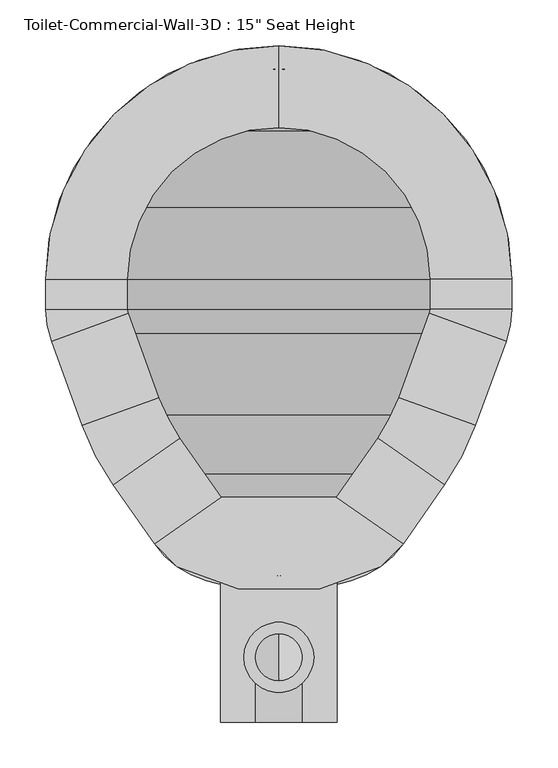
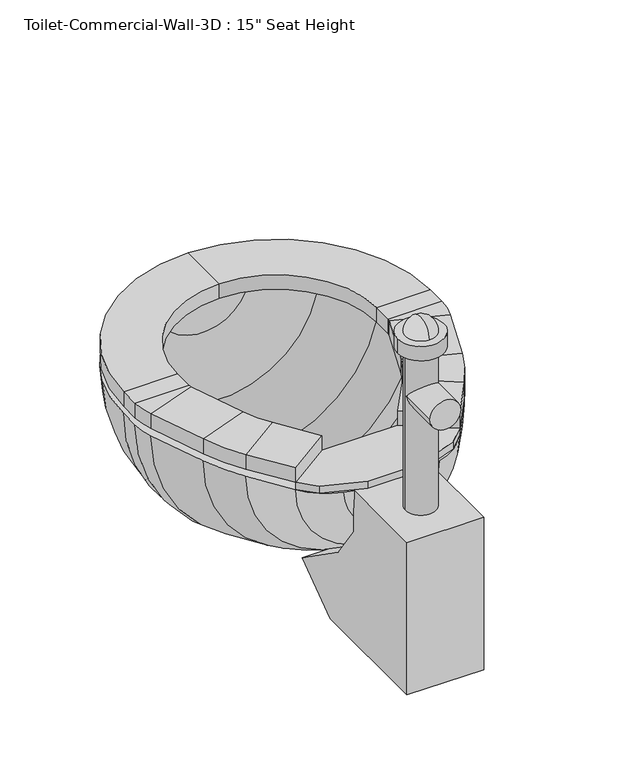
"""IFC4 building model written with IfcOpenShell, lengths in millimetres: flow terminal geometry."""

from ifc_helpers import new_model, si_unit, point, frame, frame_2d, origin, place, context, project, spatial, polyline, circle_curve, ellipse_curve, trimmed, segment, composite_curve, outline, extrude, source, transform, mapped, element, save
from ifc_brep_helpers import plane_surface, cylinder_surface, revolved_surface, advanced_brep


def flow_terminal_a02a0911(model_context):
    return source(origin(), model_context, "Body", "SolidModel", [
        extrude(outline(polyline([(216.3037941, 342.9), (216.3037941, 269.296452), (260.0103185, 206.8770663), (364.0426282, 134.0328588), (283.5454017, 76.2), (63.5, 76.2), (63.5, 342.9), (216.3037941, 342.9)])), frame((341.4031538, 0.0, 0.0), z_axis=(1.0, 0.0, 0.0), x_axis=(0.0, 1.0, 0.0)), (0.0, 0.0, 1.0), 127.0),
        extrude(outline(composite_curve([segment(trimmed(circle_curve(frame_2d((404.9031538, 134.0352737)), 25.4), [point((379.5031538, 134.0352737))], [point((430.3031538, 134.0352737))], False, "CARTESIAN"), True, "CONTINUOUS"), segment(trimmed(circle_curve(frame_2d((404.9031538, 134.0352737)), 25.4), [point((430.3031538, 134.0352737))], [point((379.5031538, 134.0352737))], False, "CARTESIAN"), True, "CONTINUOUS")], self_intersect=False)), frame((0.0, 0.0, 342.9), z_axis=(0.0, 0.0, 1.0), x_axis=(1.0, 0.0, 0.0)), (0.0, 0.0, 1.0), 279.4),
        extrude(outline(composite_curve([segment(trimmed(circle_curve(frame_2d((544.2113641, 404.9031538)), 25.4), [point((544.2113641, 379.5031538))], [point((544.2113641, 430.3031538))], False, "CARTESIAN"), True, "CONTINUOUS"), segment(trimmed(circle_curve(frame_2d((544.2113641, 404.9031538)), 25.4), [point((544.2113641, 430.3031538))], [point((544.2113641, 379.5031538))], False, "CARTESIAN"), True, "CONTINUOUS")], self_intersect=False)), frame((0.0, 63.5, 0.0), z_axis=(0.0, 1.0, 0.0), x_axis=(0.0, 0.0, 1.0)), (0.0, 0.0, 1.0), 70.64375),
        extrude(outline(composite_curve([segment(trimmed(circle_curve(frame_2d((404.9031538, 134.0352737)), 38.1), [point((366.8031538, 134.0352737))], [point((443.0031538, 134.0352737))], False, "CARTESIAN"), True, "CONTINUOUS"), segment(trimmed(circle_curve(frame_2d((404.9031538, 134.0352737)), 38.1), [point((443.0031538, 134.0352737))], [point((366.8031538, 134.0352737))], False, "CARTESIAN"), True, "CONTINUOUS")], self_intersect=False)), frame((0.0, 0.0, 622.3), z_axis=(0.0, 0.0, 1.0), x_axis=(1.0, 0.0, 0.0)), (0.0, 0.0, 1.0), 25.4),
        advanced_brep(
        [(404.9031538, 108.4176912, 647.7), (404.9031538, 159.6528563, 647.7), (404.9031538, 134.0352737, 673.3175826), (404.9031538, 134.0352737, 647.7)],
        [
            (0, 1, circle_curve(frame((404.9031538, 134.0352737, 647.7), z_axis=(0.0, 0.0, 1.0), x_axis=(0.0, 1.0, 0.0)), 25.6175826)),
            (1, 2, circle_curve(frame((404.9031538, 134.0352737, 647.7), z_axis=(1.0, 0.0, 0.0), x_axis=(0.0, -1.0, 0.0)), 25.6175826)),
            (2, 0, circle_curve(frame((404.9031538, 134.0352737, 647.7), z_axis=(1.0, 0.0, 0.0), x_axis=(0.0, 1.0, 0.0)), 25.6175826)),
            (1, 0, circle_curve(frame((404.9031538, 134.0352737, 647.7), z_axis=(0.0, 0.0, 1.0), x_axis=(0.0, 1.0, 0.0)), 25.6175826)),
            (3, 1),
            (0, 3),
        ],
        [
            revolved_surface(trimmed(ellipse_curve(frame((404.9031538, 134.0352737, 647.7), z_axis=(-1.0, 0.0, 0.0), x_axis=(0.0, -1.0, 0.0)), 25.6175826, 25.6175826), [point((404.9031538, 134.0352737, 673.3175826))], [point((404.9031538, 159.6528563, 647.7))], True, "CARTESIAN"), (404.9031538, 134.0352737, 712.3277273), (0.0, 0.0, -1.0)),
            plane_surface(frame((404.9031538, 134.0352737, 647.7), z_axis=(0.0, 0.0, -1.0), x_axis=(0.0, 1.0, 0.0))),
        ],
        [
            (0, [[1, 2, 3]]),
            (0, [[4, -3, -2]]),
            (1, [[5, -1, 6]]),
            (1, [[-6, -4, -5]]),
        ],
    ),
        advanced_brep(
        [(491.7762702, 784.7819257, 342.9), (404.9031538, 800.1, 342.9), (404.9031538, 774.7, 342.9), (483.0889586, 760.9137331, 342.9), (566.547764, 707.7446102, 342.9), (619.7168869, 624.2858048, 342.9), (633.5031538, 546.1, 342.9), (633.5031538, 513.2148212, 342.9), (628.9077315, 487.1528863, 342.9), (596.6355667, 398.4858422, 342.9), (562.9565296, 333.7890139, 342.9), (525.0728964, 279.6855786, 342.9), (468.1430637, 239.8228806, 342.9), (404.9031538, 222.8777978, 342.9), (404.9031538, 196.5817829, 342.9), (483.6469009, 217.6811063, 342.9), (540.5767337, 257.5438043, 342.9), (585.6810159, 321.9593951, 342.9), (619.360053, 386.6562234, 342.9), (652.7759241, 478.4655747, 342.9), (658.9031538, 513.2148212, 342.9), (658.9031538, 546.1, 342.9), (643.5850795, 632.9731164, 342.9), (584.5082762, 725.7051224, 342.9), (318.0300374, 784.7819257, 342.9), (225.2980314, 725.7051224, 342.9), (166.2212281, 632.9731164, 342.9), (150.9031538, 546.1, 342.9), (150.9031538, 513.2148212, 342.9), (157.0303835, 478.4655747, 342.9), (190.4462546, 386.6562234, 342.9), (224.1252917, 321.9593951, 342.9), (269.229574, 257.5438043, 342.9), (326.1594067, 217.6811063, 342.9), (341.663244, 239.8228806, 342.9), (284.7334112, 279.6855786, 342.9), (246.849778, 333.7890139, 342.9), (213.1707409, 398.4858422, 342.9), (180.8985761, 487.1528863, 342.9), (176.3031538, 513.2148212, 342.9), (176.3031538, 546.1, 342.9), (190.0894207, 624.2858048, 342.9), (243.2585436, 707.7446102, 342.9), (326.7173491, 760.9137331, 342.9)],
        [
            (0, 1, circle_curve(frame((404.9031538, 546.1, 342.9), z_axis=(0.0, 0.0, 1.0), x_axis=(1.0, 0.0, 0.0)), 254.0)),
            (1, 2),
            (2, 3, circle_curve(frame((404.9031538, 546.1, 342.9), z_axis=(0.0, 0.0, -1.0), x_axis=(1.0, 0.0, 0.0)), 228.6)),
            (3, 4, circle_curve(frame((404.9031538, 546.1, 342.9), z_axis=(0.0, 0.0, -1.0), x_axis=(1.0, 0.0, 0.0)), 228.6)),
            (4, 5, circle_curve(frame((404.9031538, 546.1, 342.9), z_axis=(0.0, 0.0, -1.0), x_axis=(1.0, 0.0, 0.0)), 228.6)),
            (5, 6, circle_curve(frame((404.9031538, 546.1, 342.9), z_axis=(0.0, 0.0, -1.0), x_axis=(1.0, 0.0, 0.0)), 228.6)),
            (6, 7),
            (7, 8, circle_curve(frame((557.3031538, 513.2148212, 342.9), z_axis=(0.0, 0.0, -1.0), x_axis=(1.0, 0.0, 0.0)), 76.2)),
            (8, 9),
            (9, 10, circle_curve(frame((334.0854485, 494.0462703, 342.9), z_axis=(0.0, 0.0, -1.0), x_axis=(1.0, 0.0, 0.0)), 279.4)),
            (10, 11),
            (11, 12, circle_curve(frame((441.8470487, 337.9609446, 342.9), z_axis=(0.0, 0.0, -1.0), x_axis=(1.0, 0.0, 0.0)), 101.6)),
            (12, 13),
            (13, 14),
            (14, 15),
            (15, 16, circle_curve(frame((457.350886, 315.8191703, 342.9), z_axis=(0.0, 0.0, 1.0), x_axis=(1.0, 0.0, 0.0)), 101.6)),
            (16, 17),
            (17, 18, circle_curve(frame((356.8099347, 482.2166514, 342.9), z_axis=(0.0, 0.0, 1.0), x_axis=(1.0, 0.0, 0.0)), 279.4)),
            (18, 19),
            (19, 20, circle_curve(frame((557.3031538, 513.2148212, 342.9), z_axis=(0.0, 0.0, 1.0), x_axis=(1.0, 0.0, 0.0)), 101.6)),
            (20, 21),
            (21, 22, circle_curve(frame((404.9031538, 546.1, 342.9), z_axis=(0.0, 0.0, 1.0), x_axis=(1.0, 0.0, 0.0)), 254.0)),
            (22, 23, circle_curve(frame((404.9031538, 546.1, 342.9), z_axis=(0.0, 0.0, 1.0), x_axis=(1.0, 0.0, 0.0)), 254.0)),
            (23, 0, circle_curve(frame((404.9031538, 546.1, 342.9), z_axis=(0.0, 0.0, 1.0), x_axis=(1.0, 0.0, 0.0)), 254.0)),
            (24, 25, circle_curve(frame((404.9031538, 546.1, 342.9), z_axis=(0.0, 0.0, 1.0), x_axis=(-1.0, 0.0, 0.0)), 254.0)),
            (25, 26, circle_curve(frame((404.9031538, 546.1, 342.9), z_axis=(0.0, 0.0, 1.0), x_axis=(-1.0, 0.0, 0.0)), 254.0)),
            (26, 27, circle_curve(frame((404.9031538, 546.1, 342.9), z_axis=(0.0, 0.0, 1.0), x_axis=(-1.0, 0.0, 0.0)), 254.0)),
            (27, 28),
            (28, 29, circle_curve(frame((252.5031538, 513.2148212, 342.9), z_axis=(0.0, 0.0, 1.0), x_axis=(-1.0, 0.0, 0.0)), 101.6)),
            (29, 30),
            (30, 31, circle_curve(frame((452.9963729, 482.2166514, 342.9), z_axis=(0.0, 0.0, 1.0), x_axis=(-1.0, 0.0, 0.0)), 279.4)),
            (31, 32),
            (32, 33, circle_curve(frame((352.4554217, 315.8191703, 342.9), z_axis=(0.0, 0.0, 1.0), x_axis=(-1.0, 0.0, 0.0)), 101.6)),
            (33, 14),
            (13, 34),
            (34, 35, circle_curve(frame((367.9592589, 337.9609446, 342.9), z_axis=(0.0, 0.0, -1.0), x_axis=(-1.0, 0.0, 0.0)), 101.6)),
            (35, 36),
            (36, 37, circle_curve(frame((475.7208592, 494.0462703, 342.9), z_axis=(0.0, 0.0, -1.0), x_axis=(-1.0, 0.0, 0.0)), 279.4)),
            (37, 38),
            (38, 39, circle_curve(frame((252.5031538, 513.2148212, 342.9), z_axis=(0.0, 0.0, -1.0), x_axis=(-1.0, 0.0, 0.0)), 76.2)),
            (39, 40),
            (40, 41, circle_curve(frame((404.9031538, 546.1, 342.9), z_axis=(0.0, 0.0, -1.0), x_axis=(-1.0, 0.0, 0.0)), 228.6)),
            (41, 42, circle_curve(frame((404.9031538, 546.1, 342.9), z_axis=(0.0, 0.0, -1.0), x_axis=(-1.0, 0.0, 0.0)), 228.6)),
            (42, 43, circle_curve(frame((404.9031538, 546.1, 342.9), z_axis=(0.0, 0.0, -1.0), x_axis=(-1.0, 0.0, 0.0)), 228.6)),
            (43, 2, circle_curve(frame((404.9031538, 546.1, 342.9), z_axis=(0.0, 0.0, -1.0), x_axis=(-1.0, 0.0, 0.0)), 228.6)),
            (1, 24, circle_curve(frame((404.9031538, 546.1, 342.9), z_axis=(0.0, 0.0, 1.0), x_axis=(-1.0, 0.0, 0.0)), 254.0)),
            (0, 24, circle_curve(frame((404.9031538, 784.7819257, 342.9), z_axis=(0.0, 1.0, 0.0), x_axis=(1.0, 0.0, 0.0)), 86.8731164)),
            (43, 3, circle_curve(frame((404.9031538, 760.9137331, 342.9), z_axis=(0.0, -1.0, 0.0), x_axis=(1.0, 0.0, 0.0)), 78.1858048)),
            (42, 4, circle_curve(frame((404.9031538, 707.7446102, 342.9), z_axis=(0.0, -1.0, 0.0), x_axis=(1.0, 0.0, 0.0)), 161.6446102)),
            (41, 5, circle_curve(frame((404.9031538, 624.2858048, 342.9), z_axis=(0.0, -1.0, 0.0), x_axis=(1.0, 0.0, 0.0)), 214.8137331)),
            (40, 6, circle_curve(frame((404.9031538, 546.1, 342.9), z_axis=(0.0, -1.0, 0.0), x_axis=(1.0, 0.0, 0.0)), 228.6)),
            (39, 7, circle_curve(frame((404.9031538, 513.2148212, 342.9), z_axis=(0.0, -1.0, 0.0), x_axis=(1.0, 0.0, 0.0)), 228.6)),
            (38, 8, circle_curve(frame((404.9031538, 487.1528863, 342.9), z_axis=(0.0, -1.0, 0.0), x_axis=(1.0, 0.0, 0.0)), 224.0045777)),
            (37, 9, circle_curve(frame((404.9031538, 398.4858422, 342.9), z_axis=(0.0, -1.0, 0.0), x_axis=(1.0, 0.0, 0.0)), 191.7324129)),
            (36, 10, circle_curve(frame((404.9031538, 333.7890139, 342.9), z_axis=(0.0, -1.0, 0.0), x_axis=(1.0, 0.0, 0.0)), 158.0533758)),
            (35, 11, circle_curve(frame((404.9031538, 279.6855786, 342.9), z_axis=(0.0, -1.0, 0.0), x_axis=(1.0, 0.0, 0.0)), 120.1697426)),
            (34, 12, circle_curve(frame((404.9031538, 239.8228806, 342.9), z_axis=(0.0, -1.0, 0.0), x_axis=(1.0, 0.0, 0.0)), 63.2399099)),
            (33, 15, circle_curve(frame((404.9031538, 217.6811063, 342.9), z_axis=(0.0, -1.0, 0.0), x_axis=(1.0, 0.0, 0.0)), 78.7437471)),
            (32, 16, circle_curve(frame((404.9031538, 257.5438043, 342.9), z_axis=(0.0, -1.0, 0.0), x_axis=(1.0, 0.0, 0.0)), 135.6735798)),
            (31, 17, circle_curve(frame((404.9031538, 321.9593951, 342.9), z_axis=(0.0, -1.0, 0.0), x_axis=(1.0, 0.0, 0.0)), 180.7778621)),
            (30, 18, circle_curve(frame((404.9031538, 386.6562234, 342.9), z_axis=(0.0, -1.0, 0.0), x_axis=(1.0, 0.0, 0.0)), 214.4568992)),
            (29, 19, circle_curve(frame((404.9031538, 478.4655747, 342.9), z_axis=(0.0, -1.0, 0.0), x_axis=(1.0, 0.0, 0.0)), 247.8727703)),
            (28, 20, circle_curve(frame((404.9031538, 513.2148212, 342.9), z_axis=(0.0, -1.0, 0.0), x_axis=(1.0, 0.0, 0.0)), 254.0)),
            (27, 21, circle_curve(frame((404.9031538, 546.1, 342.9), z_axis=(0.0, -1.0, 0.0), x_axis=(1.0, 0.0, 0.0)), 254.0)),
            (26, 22, circle_curve(frame((404.9031538, 632.9731164, 342.9), z_axis=(0.0, -1.0, 0.0), x_axis=(1.0, 0.0, 0.0)), 238.6819257)),
            (25, 23, circle_curve(frame((404.9031538, 725.7051224, 342.9), z_axis=(0.0, -1.0, 0.0), x_axis=(1.0, 0.0, 0.0)), 179.6051224)),
        ],
        [
            plane_surface(frame((404.9031538, 905.3102448, 342.9), z_axis=(0.0, 0.0, 1.0), x_axis=(1.0, 0.0, 0.0))),
            plane_surface(frame((404.9031538, 905.3102448, 342.9), z_axis=(0.0, 0.0, 1.0), x_axis=(-1.0, 0.0, 0.0))),
            revolved_surface(trimmed(ellipse_curve(frame((404.9031538, 546.1, 342.9), z_axis=(0.0, 0.0, 1.0), x_axis=(1.0, 0.0, 0.0)), 254.0, 254.0), [point((491.7762702, 784.7819257, 342.9))], [point((404.9031538, 800.1, 342.9))], True, "CARTESIAN"), (404.9031538, 905.3102448, 342.9), (0.0, 1.0, 0.0)),
            revolved_surface(trimmed(ellipse_curve(frame((404.9031538, 546.1, 342.9), z_axis=(0.0, 0.0, -1.0), x_axis=(1.0, 0.0, 0.0)), 228.6, 228.6), [point((404.9031538, 774.7, 342.9))], [point((483.0889586, 760.9137331, 342.9))], True, "CARTESIAN"), (404.9031538, 905.3102448, 342.9), (0.0, 1.0, 0.0)),
            revolved_surface(trimmed(ellipse_curve(frame((404.9031538, 546.1, 342.9), z_axis=(0.0, 0.0, -1.0), x_axis=(1.0, 0.0, 0.0)), 228.6, 228.6), [point((483.0889586, 760.9137331, 342.9))], [point((566.547764, 707.7446102, 342.9))], True, "CARTESIAN"), (404.9031538, 905.3102448, 342.9), (0.0, 1.0, 0.0)),
            revolved_surface(trimmed(ellipse_curve(frame((404.9031538, 546.1, 342.9), z_axis=(0.0, 0.0, -1.0), x_axis=(1.0, 0.0, 0.0)), 228.6, 228.6), [point((566.547764, 707.7446102, 342.9))], [point((619.7168869, 624.2858048, 342.9))], True, "CARTESIAN"), (404.9031538, 905.3102448, 342.9), (0.0, 1.0, 0.0)),
            revolved_surface(trimmed(ellipse_curve(frame((404.9031538, 546.1, 342.9), z_axis=(0.0, 0.0, -1.0), x_axis=(1.0, 0.0, 0.0)), 228.6, 228.6), [point((619.7168869, 624.2858048, 342.9))], [point((633.5031538, 546.1, 342.9))], True, "CARTESIAN"), (404.9031538, 905.3102448, 342.9), (0.0, 1.0, 0.0)),
            revolved_surface(polyline([(633.5031538, 546.1, 342.9), (633.5031538, 513.2148212, 342.9)]), (404.9031538, 905.3102448, 342.9), (0.0, 1.0, 0.0)),
            revolved_surface(trimmed(ellipse_curve(frame((557.3031538, 513.2148212, 342.9), z_axis=(0.0, 0.0, -1.0), x_axis=(1.0, 0.0, 0.0)), 76.2, 76.2), [point((633.5031538, 513.2148212, 342.9))], [point((628.9077315, 487.1528863, 342.9))], True, "CARTESIAN"), (404.9031538, 905.3102448, 342.9), (0.0, 1.0, 0.0)),
            revolved_surface(polyline([(628.9077315, 487.1528863, 342.9), (596.6355667, 398.4858422, 342.9)]), (404.9031538, 905.3102448, 342.9), (0.0, 1.0, 0.0)),
            revolved_surface(trimmed(ellipse_curve(frame((334.0854485, 494.0462703, 342.9), z_axis=(0.0, 0.0, -1.0), x_axis=(1.0, 0.0, 0.0)), 279.4, 279.4), [point((596.6355667, 398.4858422, 342.9))], [point((562.9565296, 333.7890139, 342.9))], True, "CARTESIAN"), (404.9031538, 905.3102448, 342.9), (0.0, 1.0, 0.0)),
            revolved_surface(polyline([(562.9565296, 333.7890139, 342.9), (525.0728964, 279.6855786, 342.9)]), (404.9031538, 905.3102448, 342.9), (0.0, 1.0, 0.0)),
            revolved_surface(trimmed(ellipse_curve(frame((441.8470487, 337.9609446, 342.9), z_axis=(0.0, 0.0, -1.0), x_axis=(1.0, 0.0, 0.0)), 101.6, 101.6), [point((525.0728964, 279.6855786, 342.9))], [point((468.1430637, 239.8228806, 342.9))], True, "CARTESIAN"), (404.9031538, 905.3102448, 342.9), (0.0, 1.0, 0.0)),
            revolved_surface(polyline([(468.1430637, 239.8228806, 342.9), (404.9031538, 222.8777978, 342.9)]), (404.9031538, 905.3102448, 342.9), (0.0, 1.0, 0.0)),
            revolved_surface(polyline([(404.9031538, 196.5817829, 342.9), (483.6469009, 217.6811063, 342.9)]), (404.9031538, 905.3102448, 342.9), (0.0, 1.0, 0.0)),
            revolved_surface(trimmed(ellipse_curve(frame((457.350886, 315.8191703, 342.9), z_axis=(0.0, 0.0, 1.0), x_axis=(1.0, 0.0, 0.0)), 101.6, 101.6), [point((483.6469009, 217.6811063, 342.9))], [point((540.5767337, 257.5438043, 342.9))], True, "CARTESIAN"), (404.9031538, 905.3102448, 342.9), (0.0, 1.0, 0.0)),
            revolved_surface(polyline([(540.5767337, 257.5438043, 342.9), (585.6810159, 321.9593951, 342.9)]), (404.9031538, 905.3102448, 342.9), (0.0, 1.0, 0.0)),
            revolved_surface(trimmed(ellipse_curve(frame((356.8099347, 482.2166514, 342.9), z_axis=(0.0, 0.0, 1.0), x_axis=(1.0, 0.0, 0.0)), 279.4, 279.4), [point((585.6810159, 321.9593951, 342.9))], [point((619.360053, 386.6562234, 342.9))], True, "CARTESIAN"), (404.9031538, 905.3102448, 342.9), (0.0, 1.0, 0.0)),
            revolved_surface(polyline([(619.360053, 386.6562234, 342.9), (652.7759241, 478.4655747, 342.9)]), (404.9031538, 905.3102448, 342.9), (0.0, 1.0, 0.0)),
            revolved_surface(trimmed(ellipse_curve(frame((557.3031538, 513.2148212, 342.9), z_axis=(0.0, 0.0, 1.0), x_axis=(1.0, 0.0, 0.0)), 101.6, 101.6), [point((652.7759241, 478.4655747, 342.9))], [point((658.9031538, 513.2148212, 342.9))], True, "CARTESIAN"), (404.9031538, 905.3102448, 342.9), (0.0, 1.0, 0.0)),
            cylinder_surface(frame((404.9031538, 905.3102448, 342.9), z_axis=(0.0, 1.0, 0.0), x_axis=(1.0, 0.0, 0.0)), 254.0),
            revolved_surface(trimmed(ellipse_curve(frame((404.9031538, 546.1, 342.9), z_axis=(0.0, 0.0, 1.0), x_axis=(1.0, 0.0, 0.0)), 254.0, 254.0), [point((658.9031538, 546.1, 342.9))], [point((643.5850795, 632.9731164, 342.9))], True, "CARTESIAN"), (404.9031538, 905.3102448, 342.9), (0.0, 1.0, 0.0)),
            revolved_surface(trimmed(ellipse_curve(frame((404.9031538, 546.1, 342.9), z_axis=(0.0, 0.0, 1.0), x_axis=(1.0, 0.0, 0.0)), 254.0, 254.0), [point((643.5850795, 632.9731164, 342.9))], [point((584.5082762, 725.7051224, 342.9))], True, "CARTESIAN"), (404.9031538, 905.3102448, 342.9), (0.0, 1.0, 0.0)),
            revolved_surface(trimmed(ellipse_curve(frame((404.9031538, 546.1, 342.9), z_axis=(0.0, 0.0, 1.0), x_axis=(1.0, 0.0, 0.0)), 254.0, 254.0), [point((584.5082762, 725.7051224, 342.9))], [point((491.7762702, 784.7819257, 342.9))], True, "CARTESIAN"), (404.9031538, 905.3102448, 342.9), (0.0, 1.0, 0.0)),
        ],
        [
            (0, [[1, 2, 3, 4, 5, 6, 7, 8, 9, 10, 11, 12, 13, 14, 15, 16, 17, 18, 19, 20, 21, 22, 23, 24]]),
            (1, [[25, 26, 27, 28, 29, 30, 31, 32, 33, 34, -14, 35, 36, 37, 38, 39, 40, 41, 42, 43, 44, 45, -2, 46]]),
            (2, [[-1, 47, -46]]),
            (3, [[48, -3, -45]]),
            (4, [[49, -4, -48, -44]]),
            (5, [[50, -5, -49, -43]]),
            (6, [[51, -6, -50, -42]]),
            (7, [[52, -7, -51, -41]]),
            (8, [[53, -8, -52, -40]]),
            (9, [[54, -9, -53, -39]]),
            (10, [[55, -10, -54, -38]]),
            (11, [[56, -11, -55, -37]]),
            (12, [[57, -12, -56, -36]]),
            (13, [[-13, -57, -35]]),
            (14, [[58, -15, -34]]),
            (15, [[59, -16, -58, -33]]),
            (16, [[60, -17, -59, -32]]),
            (17, [[61, -18, -60, -31]]),
            (18, [[62, -19, -61, -30]]),
            (19, [[63, -20, -62, -29]]),
            (20, [[64, -21, -63, -28]]),
            (21, [[65, -22, -64, -27]]),
            (22, [[66, -23, -65, -26]]),
            (23, [[-47, -24, -66, -25]]),
        ],
    ),
        advanced_brep(
        [(467.7541169, 308.5347495, 355.6), (540.5767337, 257.5438043, 355.6), (540.5767337, 257.5438043, 381.0), (467.7541169, 308.5347495, 381.0), (512.8583992, 372.9503403, 355.6), (585.6810159, 321.9593951, 355.6), (585.6810159, 321.9593951, 381.0), (512.8583992, 372.9503403, 381.0), (619.360053, 386.6562234, 355.6), (535.821379, 417.0618141, 355.6), (619.360053, 386.6562234, 381.0), (535.821379, 417.0618141, 381.0), (569.2372501, 508.8711654, 355.6), (652.7759241, 478.4655747, 355.6), (652.7759241, 478.4655747, 381.0), (569.2372501, 508.8711654, 381.0), (658.9031538, 513.2148212, 355.6), (570.0031538, 513.2148212, 355.6), (658.9031538, 513.2148212, 381.0), (570.0031538, 513.2148212, 381.0), (570.0031538, 546.1, 355.6), (658.9031538, 546.1, 355.6), (658.9031538, 546.1, 381.0), (570.0031538, 546.1, 381.0), (404.9031538, 800.1, 355.6), (404.9031538, 711.2, 355.6), (404.9031538, 800.1, 381.0), (404.9031538, 711.2, 381.0), (150.9031538, 546.1, 355.6), (239.8031538, 546.1, 355.6), (150.9031538, 546.1, 381.0), (239.8031538, 546.1, 381.0), (239.8031538, 513.2148212, 355.6), (150.9031538, 513.2148212, 355.6), (150.9031538, 513.2148212, 381.0), (239.8031538, 513.2148212, 381.0), (157.0303835, 478.4655747, 355.6), (240.5690575, 508.8711654, 355.6), (157.0303835, 478.4655747, 381.0), (240.5690575, 508.8711654, 381.0), (273.9849286, 417.0618141, 355.6), (190.4462546, 386.6562234, 355.6), (190.4462546, 386.6562234, 381.0), (273.9849286, 417.0618141, 381.0), (224.1252917, 321.9593951, 355.6), (296.9479084, 372.9503403, 355.6), (224.1252917, 321.9593951, 381.0), (296.9479084, 372.9503403, 381.0), (342.0521907, 308.5347495, 355.6), (342.0521907, 308.5347495, 381.0), (269.229574, 257.5438043, 381.0), (269.229574, 257.5438043, 355.6)],
        [
            (0, 1),
            (1, 2),
            (2, 3),
            (3, 0),
            (0, 4),
            (4, 5),
            (5, 1),
            (5, 6),
            (6, 2),
            (6, 7),
            (7, 3),
            (7, 4),
            (8, 5, circle_curve(frame((356.8099347, 482.2166514, 355.6), z_axis=(0.0, 0.0, -1.0), x_axis=(0.81915204428899, -0.5735764363510486, 0.0)), 279.4)),
            (4, 9, circle_curve(frame((356.8099347, 482.2166514, 355.6), z_axis=(0.0, 0.0, 1.0), x_axis=(0.81915204428899, -0.5735764363510486, 0.0)), 190.5)),
            (9, 8),
            (10, 6, circle_curve(frame((356.8099347, 482.2166514, 381.0), z_axis=(0.0, 0.0, -1.0), x_axis=(0.81915204428899, -0.5735764363510486, 0.0)), 279.4)),
            (8, 10),
            (11, 7, circle_curve(frame((356.8099347, 482.2166514, 381.0), z_axis=(0.0, 0.0, -1.0), x_axis=(0.81915204428899, -0.5735764363510486, 0.0)), 190.5)),
            (10, 11),
            (11, 9),
            (9, 12),
            (12, 13),
            (13, 8),
            (13, 14),
            (14, 10),
            (14, 15),
            (15, 11),
            (15, 12),
            (16, 13, circle_curve(frame((557.3031538, 513.2148212, 355.6), z_axis=(0.0, 0.0, -1.0), x_axis=(0.939692620785906, -0.34202014332567526, 0.0)), 101.6)),
            (12, 17, circle_curve(frame((557.3031538, 513.2148212, 355.6), z_axis=(0.0, 0.0, 1.0), x_axis=(0.939692620785906, -0.34202014332567526, 0.0)), 12.7)),
            (17, 16),
            (18, 14, circle_curve(frame((557.3031538, 513.2148212, 381.0), z_axis=(0.0, 0.0, -1.0), x_axis=(0.939692620785906, -0.34202014332567526, 0.0)), 101.6)),
            (16, 18),
            (19, 15, circle_curve(frame((557.3031538, 513.2148212, 381.0), z_axis=(0.0, 0.0, -1.0), x_axis=(0.939692620785906, -0.34202014332567526, 0.0)), 12.7)),
            (18, 19),
            (19, 17),
            (17, 20),
            (20, 21),
            (21, 16),
            (21, 22),
            (22, 18),
            (22, 23),
            (23, 19),
            (23, 20),
            (24, 21, circle_curve(frame((404.9031538, 546.1, 355.6), z_axis=(0.0, 0.0, -1.0), x_axis=(1.0, 0.0, 0.0)), 254.0)),
            (20, 25, circle_curve(frame((404.9031538, 546.1, 355.6), z_axis=(0.0, 0.0, 1.0), x_axis=(1.0, 0.0, 0.0)), 165.1)),
            (25, 24),
            (26, 22, circle_curve(frame((404.9031538, 546.1, 381.0), z_axis=(0.0, 0.0, -1.0), x_axis=(1.0, 0.0, 0.0)), 254.0)),
            (24, 26),
            (27, 23, circle_curve(frame((404.9031538, 546.1, 381.0), z_axis=(0.0, 0.0, -1.0), x_axis=(1.0, 0.0, 0.0)), 165.1)),
            (26, 27),
            (27, 25),
            (28, 24, circle_curve(frame((404.9031538, 546.1, 355.6), z_axis=(0.0, 0.0, -1.0), x_axis=(0.0, 1.0, 0.0)), 254.0)),
            (25, 29, circle_curve(frame((404.9031538, 546.1, 355.6), z_axis=(0.0, 0.0, 1.0), x_axis=(0.0, 1.0, 0.0)), 165.1)),
            (29, 28),
            (30, 26, circle_curve(frame((404.9031538, 546.1, 381.0), z_axis=(0.0, 0.0, -1.0), x_axis=(0.0, 1.0, 0.0)), 254.0)),
            (28, 30),
            (31, 27, circle_curve(frame((404.9031538, 546.1, 381.0), z_axis=(0.0, 0.0, -1.0), x_axis=(0.0, 1.0, 0.0)), 165.1)),
            (30, 31),
            (31, 29),
            (29, 32),
            (32, 33),
            (33, 28),
            (33, 34),
            (34, 30),
            (34, 35),
            (35, 31),
            (35, 32),
            (36, 33, circle_curve(frame((252.5031538, 513.2148212, 355.6), z_axis=(0.0, 0.0, -1.0), x_axis=(-1.0, 0.0, 0.0)), 101.6)),
            (32, 37, circle_curve(frame((252.5031538, 513.2148212, 355.6), z_axis=(0.0, 0.0, 1.0), x_axis=(-1.0, 0.0, 0.0)), 12.7)),
            (37, 36),
            (38, 34, circle_curve(frame((252.5031538, 513.2148212, 381.0), z_axis=(0.0, 0.0, -1.0), x_axis=(-1.0, 0.0, 0.0)), 101.6)),
            (36, 38),
            (39, 35, circle_curve(frame((252.5031538, 513.2148212, 381.0), z_axis=(0.0, 0.0, -1.0), x_axis=(-1.0, 0.0, 0.0)), 12.7)),
            (38, 39),
            (39, 37),
            (37, 40),
            (40, 41),
            (41, 36),
            (41, 42),
            (42, 38),
            (42, 43),
            (43, 39),
            (43, 40),
            (44, 41, circle_curve(frame((452.9963729, 482.2166514, 355.6), z_axis=(0.0, 0.0, -1.0), x_axis=(-0.9396926207859088, -0.34202014332566766, 0.0)), 279.4)),
            (40, 45, circle_curve(frame((452.9963729, 482.2166514, 355.6), z_axis=(0.0, 0.0, 1.0), x_axis=(-0.9396926207859088, -0.34202014332566766, 0.0)), 190.5)),
            (45, 44),
            (46, 42, circle_curve(frame((452.9963729, 482.2166514, 381.0), z_axis=(0.0, 0.0, -1.0), x_axis=(-0.9396926207859088, -0.34202014332566766, 0.0)), 279.4)),
            (44, 46),
            (47, 43, circle_curve(frame((452.9963729, 482.2166514, 381.0), z_axis=(0.0, 0.0, -1.0), x_axis=(-0.9396926207859088, -0.34202014332566766, 0.0)), 190.5)),
            (46, 47),
            (47, 45),
            (48, 49),
            (49, 50),
            (50, 51),
            (51, 48),
            (45, 48),
            (51, 44),
            (50, 46),
            (49, 47),
        ],
        [
            plane_surface(frame((540.5767337, 257.5438043, 439.6203184), z_axis=(-0.5735764363510379, -0.8191520442889975, 0.0), x_axis=(0.8191520442889975, -0.5735764363510379, 0.0))),
            plane_surface(frame((467.7541169, 308.5347495, 355.6), z_axis=(0.0, 0.0, -1.0000000000000002), x_axis=(0.5735764363510379, 0.8191520442889976, 0.0))),
            plane_surface(frame((540.5767337, 257.5438043, 355.6), z_axis=(0.8191520442889976, -0.5735764363510379, 0.0), x_axis=(0.5735764363510379, 0.8191520442889976, 0.0))),
            plane_surface(frame((540.5767337, 257.5438043, 381.0), z_axis=(0.0, 0.0, 1.0), x_axis=(0.5735764363510385, 0.8191520442889972, 0.0))),
            plane_surface(frame((467.7541169, 308.5347495, 381.0), z_axis=(-0.8191520442889972, 0.5735764363510385, 0.0), x_axis=(0.5735764363510385, 0.8191520442889972, 0.0))),
            plane_surface(frame((356.8099347, 482.2166514, 355.6), z_axis=(0.0, 0.0, -1.0), x_axis=(0.81915204428899, -0.5735764363510486, 0.0))),
            cylinder_surface(frame((356.8099347, 482.2166514, 342.9), z_axis=(0.0, 0.0, 1.0), x_axis=(0.81915204428899, -0.5735764363510486, 0.0)), 279.4),
            plane_surface(frame((356.8099347, 482.2166514, 381.0), z_axis=(0.0, 0.0, 1.0), x_axis=(0.81915204428899, -0.5735764363510486, 0.0))),
            revolved_surface(polyline([(512.8583991370526, 372.9503402751252, 381.0), (512.8583991370526, 372.9503402751252, 355.6)]), (356.8099347, 482.2166514, 342.9), (0.0, 0.0, 1.0)),
            plane_surface(frame((535.821379, 417.0618141, 355.6), z_axis=(0.0, 0.0, -1.0), x_axis=(0.34202014332566666, 0.9396926207859092, 0.0))),
            plane_surface(frame((619.360053, 386.6562234, 355.6), z_axis=(0.9396926207859093, -0.34202014332566616, 0.0), x_axis=(0.34202014332566616, 0.9396926207859093, 0.0))),
            plane_surface(frame((619.360053, 386.6562234, 381.0), z_axis=(0.0, 0.0, 1.0), x_axis=(0.34202014332566616, 0.9396926207859093, 0.0))),
            plane_surface(frame((535.821379, 417.0618141, 381.0), z_axis=(-0.9396926207859093, 0.34202014332566644, 0.0), x_axis=(0.34202014332566644, 0.9396926207859093, 0.0))),
            plane_surface(frame((557.3031538, 513.2148212, 355.6), z_axis=(0.0, 0.0, -1.0), x_axis=(0.939692620785906, -0.34202014332567526, 0.0))),
            cylinder_surface(frame((557.3031538, 513.2148212, 342.9), z_axis=(0.0, 0.0, 1.0), x_axis=(0.939692620785906, -0.34202014332567526, 0.0)), 101.6),
            plane_surface(frame((557.3031538, 513.2148212, 381.0), z_axis=(0.0, 0.0, 1.0), x_axis=(0.939692620785906, -0.34202014332567526, 0.0))),
            revolved_surface(polyline([(569.237250083981, 508.8711653797639, 381.0), (569.237250083981, 508.8711653797639, 355.6)]), (557.3031538, 513.2148212, 342.9), (0.0, 0.0, 1.0)),
            plane_surface(frame((570.0031538, 513.2148212, 355.6), z_axis=(0.0, 0.0, -1.0), x_axis=(0.0, 1.0, 0.0))),
            plane_surface(frame((658.9031538, 513.2148212, 355.6), z_axis=(1.0, 0.0, 0.0), x_axis=(0.0, 1.0, 0.0))),
            plane_surface(frame((658.9031538, 513.2148212, 381.0), z_axis=(0.0, 0.0, 1.0), x_axis=(0.0, 1.0, 0.0))),
            plane_surface(frame((570.0031538, 513.2148212, 381.0), z_axis=(-1.0, 0.0, 0.0), x_axis=(0.0, 1.0, 0.0))),
            plane_surface(frame((404.9031538, 546.1, 355.6), z_axis=(0.0, 0.0, -1.0), x_axis=(1.0, 0.0, 0.0))),
            cylinder_surface(frame((404.9031538, 546.1, 342.9), z_axis=(0.0, 0.0, 1.0), x_axis=(1.0, 0.0, 0.0)), 254.0),
            plane_surface(frame((404.9031538, 546.1, 381.0), z_axis=(0.0, 0.0, 1.0), x_axis=(1.0, 0.0, 0.0))),
            revolved_surface(polyline([(570.0031538, 546.1, 381.0), (570.0031538, 546.1, 355.6)]), (404.9031538, 546.1, 342.9), (0.0, 0.0, 1.0)),
            plane_surface(frame((404.9031538, 546.1, 355.6), z_axis=(0.0, 0.0, -1.0), x_axis=(0.0, 1.0, 0.0))),
            cylinder_surface(frame((404.9031538, 546.1, 342.9), z_axis=(0.0, 0.0, 1.0), x_axis=(0.0, 1.0, 0.0)), 254.0),
            plane_surface(frame((404.9031538, 546.1, 381.0), z_axis=(0.0, 0.0, 1.0), x_axis=(0.0, 1.0, 0.0))),
            revolved_surface(polyline([(404.9031538, 711.2, 381.0), (404.9031538, 711.2, 355.6)]), (404.9031538, 546.1, 342.9), (0.0, 0.0, 1.0)),
            plane_surface(frame((239.8031538, 546.1, 355.6), z_axis=(0.0, 0.0, -1.0), x_axis=(0.0, -1.0, 0.0))),
            plane_surface(frame((150.9031538, 546.1, 355.6), z_axis=(-1.0, 0.0, 0.0), x_axis=(0.0, -1.0, 0.0))),
            plane_surface(frame((150.9031538, 546.1, 381.0), z_axis=(0.0, 0.0, 1.0), x_axis=(0.0, -1.0, 0.0))),
            plane_surface(frame((239.8031538, 546.1, 381.0), z_axis=(1.0, 0.0, 0.0), x_axis=(0.0, -1.0, 0.0))),
            plane_surface(frame((252.5031538, 513.2148212, 355.6), z_axis=(0.0, 0.0, -1.0), x_axis=(-1.0, 0.0, 0.0))),
            cylinder_surface(frame((252.5031538, 513.2148212, 342.9), z_axis=(0.0, 0.0, 1.0), x_axis=(-1.0, 0.0, 0.0)), 101.6),
            plane_surface(frame((252.5031538, 513.2148212, 381.0), z_axis=(0.0, 0.0, 1.0), x_axis=(-1.0, 0.0, 0.0))),
            revolved_surface(polyline([(239.80315380000002, 513.2148212, 381.0), (239.80315380000002, 513.2148212, 355.6)]), (252.5031538, 513.2148212, 342.9), (0.0, 0.0, 1.0)),
            plane_surface(frame((240.5690575, 508.8711654, 355.6), z_axis=(0.0, 0.0, -1.0), x_axis=(0.34202014332565583, -0.9396926207859131, 0.0))),
            plane_surface(frame((157.0303835, 478.4655747, 355.6), z_axis=(-0.9396926207859133, -0.34202014332565556, 0.0), x_axis=(0.34202014332565556, -0.9396926207859133, 0.0))),
            plane_surface(frame((157.0303835, 478.4655747, 381.0), z_axis=(0.0, 0.0, 1.0), x_axis=(0.34202014332565583, -0.9396926207859131, 0.0))),
            plane_surface(frame((240.5690575, 508.8711654, 381.0), z_axis=(0.9396926207859132, 0.3420201433256555, 0.0), x_axis=(0.3420201433256555, -0.9396926207859132, 0.0))),
            plane_surface(frame((452.9963729, 482.2166514, 355.6), z_axis=(0.0, 0.0, -1.0), x_axis=(-0.9396926207859088, -0.34202014332566766, 0.0))),
            cylinder_surface(frame((452.9963729, 482.2166514, 342.9), z_axis=(0.0, 0.0, 1.0), x_axis=(-0.9396926207859088, -0.34202014332566766, 0.0)), 279.4),
            plane_surface(frame((452.9963729, 482.2166514, 381.0), z_axis=(0.0, 0.0, 1.0), x_axis=(-0.9396926207859088, -0.34202014332566766, 0.0))),
            revolved_surface(polyline([(273.98492864028435, 417.0618140964603, 381.0), (273.98492864028435, 417.0618140964603, 355.6)]), (452.9963729, 482.2166514, 342.9), (0.0, 0.0, 1.0)),
            plane_surface(frame((269.229574, 257.5438043, 246.1796816), z_axis=(0.5735764363510504, -0.8191520442889889, 0.0), x_axis=(0.8191520442889889, 0.5735764363510504, 0.0))),
            plane_surface(frame((296.9479084, 372.9503403, 355.6), z_axis=(0.0, 0.0, -1.0), x_axis=(0.5735764363510505, -0.8191520442889888, 0.0))),
            plane_surface(frame((224.1252917, 321.9593951, 355.6), z_axis=(-0.8191520442889885, -0.5735764363510509, 0.0), x_axis=(0.5735764363510509, -0.8191520442889885, 0.0))),
            plane_surface(frame((224.1252917, 321.9593951, 381.0), z_axis=(0.0, 0.0, 1.0000000000000002), x_axis=(0.5735764363510502, -0.819152044288989, 0.0))),
            plane_surface(frame((296.9479084, 372.9503403, 381.0), z_axis=(0.8191520442889887, 0.5735764363510507, 0.0), x_axis=(0.5735764363510507, -0.8191520442889887, 0.0))),
        ],
        [
            (0, [[1, 2, 3, 4]]),
            (1, [[-1, 5, 6, 7]]),
            (2, [[-2, -7, 8, 9]]),
            (3, [[-3, -9, 10, 11]]),
            (4, [[-4, -11, 12, -5]]),
            (5, [[13, -6, 14, 15]]),
            (6, [[16, -8, -13, 17]]),
            (7, [[18, -10, -16, 19]]),
            (8, [[-14, -12, -18, 20]]),
            (9, [[-15, 21, 22, 23]]),
            (10, [[-17, -23, 24, 25]]),
            (11, [[-19, -25, 26, 27]]),
            (12, [[-20, -27, 28, -21]]),
            (13, [[29, -22, 30, 31]]),
            (14, [[32, -24, -29, 33]]),
            (15, [[34, -26, -32, 35]]),
            (16, [[-30, -28, -34, 36]]),
            (17, [[-31, 37, 38, 39]]),
            (18, [[-33, -39, 40, 41]]),
            (19, [[-35, -41, 42, 43]]),
            (20, [[-36, -43, 44, -37]]),
            (21, [[45, -38, 46, 47]]),
            (22, [[48, -40, -45, 49]]),
            (23, [[50, -42, -48, 51]]),
            (24, [[-46, -44, -50, 52]]),
            (25, [[53, -47, 54, 55]]),
            (26, [[56, -49, -53, 57]]),
            (27, [[58, -51, -56, 59]]),
            (28, [[-54, -52, -58, 60]]),
            (29, [[-55, 61, 62, 63]]),
            (30, [[-57, -63, 64, 65]]),
            (31, [[-59, -65, 66, 67]]),
            (32, [[-60, -67, 68, -61]]),
            (33, [[69, -62, 70, 71]]),
            (34, [[72, -64, -69, 73]]),
            (35, [[74, -66, -72, 75]]),
            (36, [[-70, -68, -74, 76]]),
            (37, [[-71, 77, 78, 79]]),
            (38, [[-73, -79, 80, 81]]),
            (39, [[-75, -81, 82, 83]]),
            (40, [[-76, -83, 84, -77]]),
            (41, [[85, -78, 86, 87]]),
            (42, [[88, -80, -85, 89]]),
            (43, [[90, -82, -88, 91]]),
            (44, [[-86, -84, -90, 92]]),
            (45, [[93, 94, 95, 96]]),
            (46, [[-87, 97, -96, 98]]),
            (47, [[-89, -98, -95, 99]]),
            (48, [[-91, -99, -94, 100]]),
            (49, [[-92, -100, -93, -97]]),
        ],
    ),
        extrude(outline(polyline([(467.7541169, 308.5347495), (540.5767337, 257.5438043), (515.6262519, 232.5933226), (449.563909, 208.5485961), (360.2423986, 208.5485961), (294.1800557, 232.5933226), (269.229574, 257.5438043), (342.0521907, 308.5347495), (467.7541169, 308.5347495)])), frame((0.0, 0.0, 342.9), z_axis=(0.0, 0.0, 1.0), x_axis=(1.0, 0.0, 0.0)), (0.0, 0.0, 1.0), 12.7),
    ])


if __name__ == "__main__":
    model = new_model("IFC4")
    model_context = context("Model", 3, world=origin())
    ifc_project = project(units=[si_unit("LENGTHUNIT", "METRE", prefix="MILLI")], contexts=[model_context])
    site = spatial("IfcSite", under=ifc_project)
    building = spatial("IfcBuilding", under=site)
    placement = place(None, origin())
    flow_terminal_shape = flow_terminal_a02a0911(model_context)
    element("IfcFlowTerminal", 1, ObjectType="Toilet-Commercial-Wall-3D : 15\" Seat Height", at=placement, inside=building, context=model_context, shape_type="MappedRepresentation", body=[
        mapped(flow_terminal_shape, transform((0.0, 0.0, 0.0), x_axis=(1.0, 0.0, 0.0), y_axis=(0.0, 1.0, 0.0), z_axis=(0.0, 0.0, 1.0))),
    ])
    save(model, "model.ifc")

# Revit data of these elements
# Type "Toilet-Commercial-Wall-3D : 15\" Seat Height"
#   Assembly Code = "D2010110"
#   Mounting Height = 1' - 3"
#   Piping Material = Steel, Polished
#   Toilet - Bowl Material = Porcelain, Ivory
#   Toilet - Seat Material = Laminate, Ivory, Matte
#   Default Elevation = 0
# Element 1 (IfcFlowTerminal, "Toilet-Commercial-Wall-3D : 15\" Seat Height")
#   Materials on its faces: "Laminate, Ivory, Matte", "Porcelain, Ivory", "Steel, Polished"
# Materials
#   "Steel, Polished": class "Metal", colour RGB 57 57 57, transparency 0, Description = "Polished steel", Cost = 0
#   "Porcelain, Ivory": class "Ceramic", colour RGB 247 247 239, transparency 0, Description = "Porcelain, ivory", Cost = 0
#   "Laminate, Ivory, Matte": class "Plastic", colour RGB 247 247 239, transparency 0, Description = "Plastic Laminate - Ivory, Matte", Cost = 0
